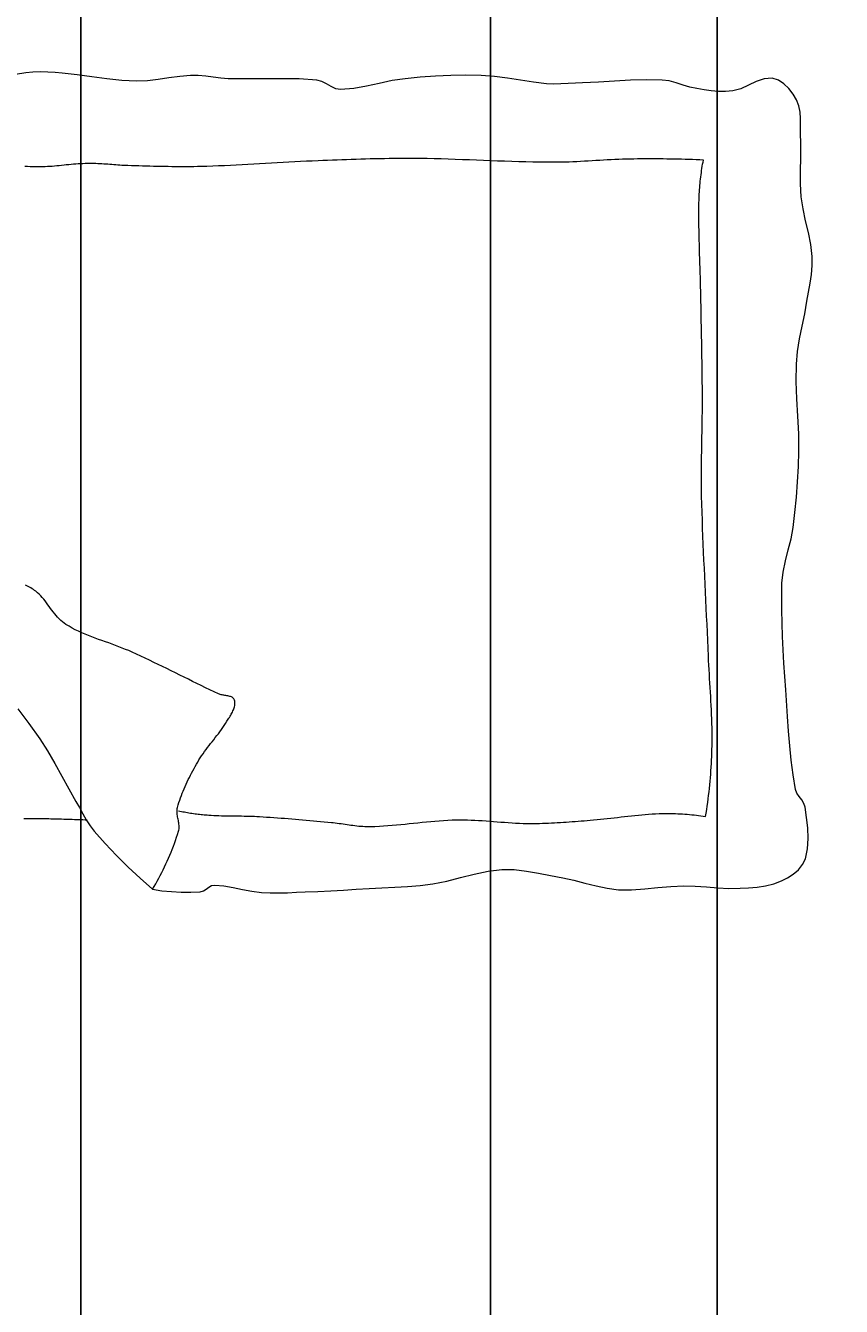
# Model space of a CAD drawing. Units: inches. Extents: x -15 to 423, y -713 to 71.
# Tile 8 of 24: x 70 to 144, y -234 to -117. Entities that reach past the tile are written whole.
import ezdxf

# ---------------------------------------------------------------- set-up
doc = ezdxf.new("R2010")
doc.units = ezdxf.units.IN
doc.header["$MEASUREMENT"] = 0
doc.layers.add('A-ANNO-DIMS', color=2, linetype='Continuous', lineweight=18)
doc.layers.add('A-FURN', color=9, linetype='Continuous', lineweight=13)
doc.styles.get("Standard").update_dxf_attribs({"font": 'arial.ttf'})
doc.dimstyles.get("Standard").update_dxf_attribs({"dimtxt": 0.18, "dimasz": 0.18, "dimexe": 0.18, "dimexo": 0.0625, "dimgap": 0.09, "dimtad": 0, "dimtih": 1, "dimtoh": 1, "dimdec": 0, "dimzin": 0, "dimdsep": 46, "dimlunit": 3, "dimtxsty": 'Standard', "dimcen": 0.09, "dimadec": 0, "dimazin": 0, "dimtfac": 1, "dimtdec": 0, "dimtofl": 0, "dimtmove": 0, "dimatfit": 3, "dimfxl": 1, "dimtolj": 1, "dimtzin": 0, "dimarcsym": 0})

# ---------------------------------------------------------------- blocks, each defined once
blk = doc.blocks.new('*D39')
at = {"layer": 'A-ANNO-DIMS', "color": 0, "lineweight": -2, "transparency": 16777216}
for p, q in [((75.05, -253.53), (75.05, 57.43)), ((75.23, 57.25), (93.19, 57.25)), ((112.22, 57.25), (94.26, 57.25)), ((112.4, -253.53), (112.4, 57.43))]:
    blk.add_line(p, q, dxfattribs=at)
at = {"layer": 'A-ANNO-DIMS', "color": 0, "transparency": 16777216}
for points in [[(75.23, 57.28), (75.23, 57.22), (75.05, 57.25)], [(112.22, 57.28), (112.22, 57.22), (112.4, 57.25)]]:
    blk.add_solid(points, dxfattribs=at)
at = {"layer": 'Defpoints', "color": 0, "transparency": 16777216}
for p in [(112.4, 57.25), (75.05, -253.59), (112.4, -253.59)]:
    blk.add_point(p, dxfattribs=at)
at = {"layer": 'A-ANNO-DIMS', "color": 0, "transparency": 16777216, "insert": (93.72, 57.25), "char_height": 0.18, "attachment_point": 5}
blk.add_mtext('\\A1;3\'-1 1/2"', dxfattribs=at)
blk = doc.blocks.new('*D42')
at = {"layer": 'A-ANNO-DIMS', "color": 0, "lineweight": -2, "transparency": 16777216}
for p, q in [((133.08, -409.94), (133.08, 57.43)), ((133.26, 57.25), (157.25, 57.25)), ((181.9, 57.25), (157.91, 57.25)), ((182.08, -409.94), (182.08, 57.43))]:
    blk.add_line(p, q, dxfattribs=at)
at = {"layer": 'A-ANNO-DIMS', "color": 0, "transparency": 16777216}
for points in [[(133.26, 57.28), (133.26, 57.22), (133.08, 57.25)], [(181.9, 57.28), (181.9, 57.22), (182.08, 57.25)]]:
    blk.add_solid(points, dxfattribs=at)
at = {"layer": 'Defpoints', "color": 0, "transparency": 16777216}
for p in [(182.08, 57.25), (133.08, -410), (182.08, -410)]:
    blk.add_point(p, dxfattribs=at)
at = {"layer": 'A-ANNO-DIMS', "color": 0, "transparency": 16777216, "insert": (157.58, 57.25), "char_height": 0.18, "attachment_point": 5}
blk.add_mtext('\\A1;4\'-1"', dxfattribs=at)

msp = doc.modelspace()

# ---------------------------------------------------------------- linework, layer by layer
at = {"layer": 'A-FURN'}
for p, q in [((70.02, -121.16), (69.09, -121.33)), ((70.68, -121.1), (70.02, -121.16)), ((71.35, -121.08), (70.68, -121.1)), ((72.02, -121.11), (71.35, -121.08)), ((72.69, -121.15), (72.02, -121.11)), ((73.35, -121.2), (72.69, -121.15)), ((74.71, -121.34), (73.35, -121.2)), ((76.06, -121.53), (74.71, -121.34)), ((85.06, -121.41), (84.07, -121.49)), ((85.74, -121.42), (85.06, -121.41)), ((86.43, -121.48), (85.74, -121.42)), ((107.39, -121.47), (106, -121.57)), ((108.78, -121.4), (107.39, -121.47)), ((110.17, -121.38), (108.78, -121.4)), ((111.57, -121.4), (110.17, -121.38)), ((112.76, -121.5), (111.57, -121.4)), ((77.41, -121.71), (76.06, -121.53)), ((78.77, -121.87), (77.41, -121.71)), ((80.13, -121.94), (78.77, -121.87)), ((81.12, -121.9), (80.13, -121.94)), ((82.1, -121.78), (81.12, -121.9)), ((83.08, -121.63), (82.1, -121.78)), ((84.07, -121.49), (83.08, -121.63)), ((87.11, -121.57), (86.43, -121.48)), ((87.8, -121.65), (87.11, -121.57)), ((88.48, -121.7), (87.8, -121.65)), ((90.1, -121.72), (88.48, -121.7)), ((91.72, -121.71), (90.1, -121.72)), ((93.34, -121.7), (91.72, -121.71)), ((94.95, -121.72), (93.34, -121.7)), ((96.56, -121.83), (94.95, -121.72)), ((97.01, -121.95), (96.56, -121.83)), ((97.44, -122.17), (97.01, -121.95)), ((97.86, -122.42), (97.44, -122.17)), ((98.29, -122.62), (97.86, -122.42)), ((98.74, -122.7), (98.29, -122.62)), ((99.93, -122.6), (98.74, -122.7)), ((101.1, -122.39), (99.93, -122.6)), ((102.26, -122.13), (101.1, -122.39)), ((103.43, -121.87), (102.26, -122.13)), ((104.61, -121.7), (103.43, -121.87)), ((106, -121.57), (104.61, -121.7)), ((113.95, -121.66), (112.76, -121.5)), ((115.13, -121.85), (113.95, -121.66)), ((116.32, -122.03), (115.13, -121.85)), ((117.52, -122.16), (116.32, -122.03)), ((118.17, -122.19), (117.52, -122.16)), ((118.83, -122.18), (118.17, -122.19)), ((119.49, -122.15), (118.83, -122.18)), ((120.15, -122.11), (119.49, -122.15)), ((120.81, -122.08), (120.15, -122.11)), ((122.26, -122.01), (120.81, -122.08)), ((123.71, -121.92), (122.26, -122.01)), ((125.16, -121.84), (123.71, -121.92)), ((126.6, -121.8), (125.16, -121.84)), ((128.05, -121.82), (126.6, -121.8)), ((128.7, -121.91), (128.05, -121.82)), ((129.34, -122.08), (128.7, -121.91)), ((129.97, -122.28), (129.34, -122.08)), ((130.6, -122.47), (129.97, -122.28)), ((131.24, -122.61), (130.6, -122.47)), ((131.89, -122.71), (131.24, -122.61)), ((135.24, -122.62), (134.5, -122.82)), ((135.95, -122.29), (135.24, -122.62)), ((136.65, -121.95), (135.95, -122.29)), ((137.37, -121.7), (136.65, -121.95)), ((138.1, -121.66), (137.37, -121.7)), ((138.66, -121.83), (138.1, -121.66)), ((139.17, -122.16), (138.66, -121.83)), ((139.63, -122.6), (139.17, -122.16)), ((140.01, -123.1), (139.63, -122.6)), ((132.54, -122.8), (131.89, -122.71)), ((133.2, -122.86), (132.54, -122.8)), ((133.85, -122.87), (133.2, -122.86)), ((134.5, -122.82), (133.85, -122.87)), ((140.33, -123.63), (140.01, -123.1)), ((140.54, -124.17), (140.33, -123.63)), ((140.64, -124.74), (140.54, -124.17)), ((140.68, -125.34), (140.64, -124.74)), ((140.68, -125.95), (140.68, -125.34)), ((140.69, -126.54), (140.68, -125.95)), ((140.71, -127.73), (140.69, -126.54)), ((140.7, -128.92), (140.71, -127.73)), ((73.08, -129.64), (72.86, -129.66)), ((73.29, -129.62), (73.08, -129.64)), ((73.51, -129.59), (73.29, -129.62)), ((73.72, -129.57), (73.51, -129.59)), ((73.94, -129.55), (73.72, -129.57)), ((74.15, -129.53), (73.94, -129.55)), ((74.37, -129.51), (74.15, -129.53)), ((74.59, -129.49), (74.37, -129.51)), ((74.8, -129.47), (74.59, -129.49)), ((75.02, -129.46), (74.8, -129.47)), ((75.23, -129.45), (75.02, -129.46)), ((75.45, -129.44), (75.23, -129.45)), ((75.67, -129.43), (75.45, -129.44)), ((75.85, -129.43), (75.67, -129.43)), ((76.03, -129.43), (75.85, -129.43)), ((76.22, -129.44), (76.03, -129.43)), ((76.4, -129.44), (76.22, -129.44)), ((76.58, -129.45), (76.4, -129.44)), ((76.77, -129.46), (76.58, -129.45)), ((76.95, -129.47), (76.77, -129.46)), ((77.13, -129.49), (76.95, -129.47)), ((77.32, -129.5), (77.13, -129.49)), ((77.5, -129.51), (77.32, -129.5)), ((77.69, -129.53), (77.5, -129.51)), ((77.87, -129.54), (77.69, -129.53)), ((78.05, -129.56), (77.87, -129.54)), ((78.24, -129.57), (78.05, -129.56)), ((78.42, -129.58), (78.24, -129.57)), ((78.6, -129.6), (78.42, -129.58)), ((78.79, -129.61), (78.6, -129.6)), ((78.97, -129.62), (78.79, -129.61)), ((79.15, -129.63), (78.97, -129.62)), ((79.34, -129.63), (79.15, -129.63)), ((79.67, -129.64), (79.34, -129.63)), ((80, -129.65), (79.67, -129.64)), ((88.15, -129.64), (87.61, -129.66)), ((88.68, -129.62), (88.15, -129.64)), ((89.22, -129.59), (88.68, -129.62)), ((89.75, -129.56), (89.22, -129.59)), ((90.28, -129.53), (89.75, -129.56)), ((90.82, -129.5), (90.28, -129.53)), ((91.35, -129.47), (90.82, -129.5)), ((91.88, -129.44), (91.35, -129.47)), ((92.42, -129.41), (91.88, -129.44)), ((92.95, -129.38), (92.42, -129.41)), ((93.49, -129.35), (92.95, -129.38)), ((94.02, -129.32), (93.49, -129.35)), ((94.55, -129.29), (94.02, -129.32)), ((95.09, -129.26), (94.55, -129.29)), ((95.62, -129.23), (95.09, -129.26)), ((96.15, -129.21), (95.62, -129.23)), ((96.69, -129.19), (96.15, -129.21)), ((97.12, -129.17), (96.69, -129.19)), ((97.55, -129.16), (97.12, -129.17)), ((97.99, -129.14), (97.55, -129.16)), ((98.42, -129.12), (97.99, -129.14)), ((98.85, -129.11), (98.42, -129.12)), ((99.28, -129.09), (98.85, -129.11)), ((99.71, -129.08), (99.28, -129.09)), ((100.15, -129.06), (99.71, -129.08)), ((100.58, -129.05), (100.15, -129.06)), ((101.01, -129.04), (100.58, -129.05)), ((101.44, -129.02), (101.01, -129.04)), ((101.88, -129.01), (101.44, -129.02)), ((102.31, -129), (101.88, -129.01)), ((102.74, -129), (102.31, -129)), ((103.17, -128.99), (102.74, -129)), ((103.6, -128.98), (103.17, -128.99)), ((104.04, -128.98), (103.6, -128.98)), ((104.47, -128.98), (104.04, -128.98)), ((104.9, -128.98), (104.47, -128.98)), ((105.33, -128.98), (104.9, -128.98)), ((105.98, -128.98), (105.33, -128.98)), ((106.62, -128.99), (105.98, -128.98)), ((107.26, -129.01), (106.62, -128.99)), ((107.91, -129.02), (107.26, -129.01)), ((108.55, -129.04), (107.91, -129.02)), ((109.19, -129.06), (108.55, -129.04)), ((109.84, -129.09), (109.19, -129.06)), ((110.48, -129.11), (109.84, -129.09)), ((111.12, -129.13), (110.48, -129.11)), ((111.76, -129.16), (111.12, -129.13)), ((112.41, -129.18), (111.76, -129.16)), ((113.05, -129.21), (112.41, -129.18)), ((113.69, -129.23), (113.05, -129.21)), ((114.34, -129.25), (113.69, -129.23)), ((114.98, -129.27), (114.34, -129.25)), ((115.62, -129.29), (114.98, -129.27)), ((116.26, -129.3), (115.62, -129.29)), ((116.91, -129.31), (116.26, -129.3)), ((117.55, -129.32), (116.91, -129.31)), ((118.19, -129.32), (117.55, -129.32)), ((118.54, -129.32), (118.19, -129.32)), ((118.89, -129.32), (118.54, -129.32)), ((119.24, -129.31), (118.89, -129.32)), ((119.59, -129.3), (119.24, -129.31)), ((119.93, -129.29), (119.59, -129.3)), ((120.28, -129.27), (119.93, -129.29)), ((120.63, -129.25), (120.28, -129.27)), ((120.98, -129.23), (120.63, -129.25)), ((121.32, -129.21), (120.98, -129.23)), ((121.67, -129.19), (121.32, -129.21)), ((122.02, -129.17), (121.67, -129.19)), ((122.37, -129.15), (122.02, -129.17)), ((122.71, -129.13), (122.37, -129.15)), ((123.06, -129.11), (122.71, -129.13)), ((123.41, -129.09), (123.06, -129.11)), ((123.76, -129.08), (123.41, -129.09)), ((124.11, -129.06), (123.76, -129.08)), ((124.45, -129.05), (124.11, -129.06)), ((124.8, -129.04), (124.45, -129.05)), ((125.15, -129.03), (124.8, -129.04)), ((125.48, -129.03), (125.15, -129.03)), ((125.82, -129.02), (125.48, -129.03)), ((126.15, -129.02), (125.82, -129.02)), ((126.48, -129.02), (126.15, -129.02)), ((126.82, -129.02), (126.48, -129.02)), ((127.15, -129.02), (126.82, -129.02)), ((127.49, -129.02), (127.15, -129.02)), ((127.82, -129.02), (127.49, -129.02)), ((128.15, -129.02), (127.82, -129.02)), ((128.49, -129.03), (128.15, -129.02)), ((128.82, -129.03), (128.49, -129.03)), ((129.15, -129.04), (128.82, -129.03)), ((129.49, -129.04), (129.15, -129.04)), ((129.82, -129.05), (129.49, -129.04)), ((130.16, -129.06), (129.82, -129.05)), ((130.49, -129.07), (130.16, -129.06)), ((130.82, -129.08), (130.49, -129.07)), ((131.16, -129.09), (130.82, -129.08)), ((131.49, -129.1), (131.16, -129.09)), ((131.82, -129.12), (131.49, -129.1)), ((131.72, -129.69), (131.75, -129.5)), ((131.75, -129.5), (131.79, -129.31)), ((131.79, -129.31), (131.82, -129.12)), ((140.68, -130.1), (140.7, -128.92)), ((70.18, -129.72), (69.95, -129.71)), ((70.42, -129.73), (70.18, -129.72)), ((70.65, -129.74), (70.42, -129.73)), ((70.88, -129.74), (70.65, -129.74)), ((71.12, -129.74), (70.88, -129.74)), ((71.35, -129.74), (71.12, -129.74)), ((71.56, -129.74), (71.35, -129.74)), ((71.78, -129.73), (71.56, -129.74)), ((72, -129.72), (71.78, -129.73)), ((72.21, -129.71), (72, -129.72)), ((72.43, -129.7), (72.21, -129.71)), ((72.64, -129.68), (72.43, -129.7)), ((72.86, -129.66), (72.64, -129.68)), ((80.34, -129.66), (80, -129.65)), ((80.67, -129.67), (80.34, -129.66)), ((81.01, -129.68), (80.67, -129.67)), ((81.34, -129.69), (81.01, -129.68)), ((81.67, -129.7), (81.34, -129.69)), ((82.01, -129.71), (81.67, -129.7)), ((82.34, -129.71), (82.01, -129.71)), ((82.67, -129.72), (82.34, -129.71)), ((83.01, -129.72), (82.67, -129.72)), ((83.34, -129.73), (83.01, -129.72)), ((83.68, -129.73), (83.34, -129.73)), ((84.01, -129.74), (83.68, -129.73)), ((84.34, -129.74), (84.01, -129.74)), ((84.68, -129.74), (84.34, -129.74)), ((85.01, -129.73), (84.68, -129.74)), ((85.34, -129.73), (85.01, -129.73)), ((85.68, -129.72), (85.34, -129.73)), ((86.01, -129.72), (85.68, -129.72)), ((86.55, -129.7), (86.01, -129.72)), ((87.08, -129.68), (86.55, -129.7)), ((87.61, -129.66), (87.08, -129.68)), ((131.56, -130.85), (131.59, -130.66)), ((131.59, -130.66), (131.61, -130.47)), ((131.61, -130.47), (131.64, -130.27)), ((131.64, -130.27), (131.66, -130.08)), ((131.66, -130.08), (131.69, -129.89)), ((131.69, -129.89), (131.72, -129.69)), ((140.68, -131.29), (140.68, -130.1)), ((131.46, -132.02), (131.48, -131.83)), ((131.48, -131.83), (131.49, -131.63)), ((131.49, -131.63), (131.51, -131.44)), ((131.51, -131.44), (131.52, -131.24)), ((131.52, -131.24), (131.54, -131.05)), ((131.54, -131.05), (131.56, -130.85)), ((140.75, -132.47), (140.68, -131.29)), ((131.42, -133), (131.43, -132.8)), ((131.42, -133.42), (131.42, -133)), ((131.43, -132.61), (131.44, -132.41)), ((131.43, -132.8), (131.43, -132.61)), ((131.44, -132.41), (131.45, -132.22)), ((131.45, -132.22), (131.46, -132.02)), ((140.91, -133.57), (140.75, -132.47)), ((131.41, -133.85), (131.42, -133.42)), ((131.41, -134.28), (131.41, -133.85)), ((131.42, -134.7), (131.41, -134.28)), ((141.15, -134.66), (140.91, -133.57)), ((131.42, -135.13), (131.42, -134.7)), ((131.43, -135.56), (131.42, -135.13)), ((141.4, -135.74), (141.15, -134.66)), ((131.44, -135.98), (131.43, -135.56)), ((131.45, -136.41), (131.44, -135.98)), ((131.46, -136.83), (131.45, -136.41)), ((141.62, -136.83), (141.4, -135.74)), ((131.47, -137.26), (131.46, -136.83)), ((131.48, -137.69), (131.47, -137.26)), ((131.5, -138.11), (131.48, -137.69)), ((141.75, -137.93), (141.62, -136.83)), ((131.51, -138.54), (131.5, -138.11)), ((131.52, -138.96), (131.51, -138.54)), ((131.54, -139.39), (131.52, -138.96)), ((141.67, -139.55), (141.75, -138.74)), ((141.75, -138.74), (141.75, -137.93)), ((131.55, -139.82), (131.54, -139.39)), ((131.56, -140.24), (131.55, -139.82)), ((141.55, -140.36), (141.67, -139.55)), ((131.57, -140.67), (131.56, -140.24)), ((131.58, -141.09), (131.57, -140.67)), ((131.59, -141.52), (131.58, -141.09)), ((141.27, -141.98), (141.4, -141.17)), ((141.4, -141.17), (141.55, -140.36)), ((131.6, -141.98), (131.59, -141.52)), ((131.61, -142.44), (131.6, -141.98)), ((131.62, -142.9), (131.61, -142.44)), ((141.07, -143.13), (141.27, -141.98)), ((131.62, -143.37), (131.62, -142.9)), ((131.63, -143.83), (131.62, -143.37)), ((140.84, -144.27), (141.07, -143.13)), ((131.64, -144.29), (131.63, -143.83)), ((131.65, -144.75), (131.64, -144.29)), ((131.66, -145.21), (131.65, -144.75)), ((140.6, -145.42), (140.84, -144.27)), ((131.67, -145.67), (131.66, -145.21)), ((131.68, -146.13), (131.67, -145.67)), ((140.41, -146.57), (140.6, -145.42)), ((131.68, -146.59), (131.68, -146.13)), ((131.69, -147.06), (131.68, -146.59)), ((131.7, -147.52), (131.69, -147.06)), ((140.3, -147.72), (140.41, -146.57)), ((131.71, -147.98), (131.7, -147.52)), ((131.71, -148.44), (131.71, -147.98)), ((140.27, -149.31), (140.3, -147.72)), ((131.72, -148.9), (131.71, -148.44)), ((131.72, -149.36), (131.72, -148.9)), ((131.73, -149.82), (131.72, -149.36)), ((140.34, -150.9), (140.27, -149.31)), ((131.73, -150.28), (131.73, -149.82)), ((131.73, -150.74), (131.73, -150.28)), ((131.73, -151.2), (131.73, -150.74)), ((131.73, -151.65), (131.73, -151.2)), ((131.73, -152.1), (131.73, -151.65)), ((140.43, -152.49), (140.34, -150.9)), ((131.71, -153.45), (131.72, -153)), ((131.72, -152.55), (131.73, -152.1)), ((131.72, -153), (131.72, -152.55)), ((140.52, -154.08), (140.43, -152.49)), ((131.69, -154.35), (131.7, -153.9)), ((131.7, -153.9), (131.71, -153.45)), ((140.53, -155.67), (140.52, -154.08)), ((131.67, -155.71), (131.68, -155.26)), ((131.68, -154.81), (131.69, -154.35)), ((131.68, -155.26), (131.68, -154.81)), ((131.65, -156.61), (131.66, -156.16)), ((131.66, -156.16), (131.67, -155.71)), ((140.49, -157.07), (140.53, -155.67)), ((131.65, -157.06), (131.65, -156.61)), ((131.65, -157.51), (131.65, -157.06)), ((131.65, -157.96), (131.65, -157.51)), ((140.41, -158.47), (140.49, -157.07)), ((131.65, -158.41), (131.65, -157.96)), ((131.65, -158.87), (131.65, -158.41)), ((140.3, -159.86), (140.41, -158.47)), ((131.65, -159.32), (131.65, -158.87)), ((131.66, -159.77), (131.65, -159.32)), ((131.68, -160.5), (131.66, -159.77)), ((140.17, -161.25), (140.3, -159.86)), ((131.7, -161.23), (131.68, -160.5)), ((131.73, -161.96), (131.7, -161.23)), ((131.75, -162.69), (131.73, -161.96)), ((140, -162.64), (140.17, -161.25)), ((131.78, -163.42), (131.75, -162.69)), ((131.81, -164.14), (131.78, -163.42)), ((139.82, -163.66), (140, -162.64)), ((131.84, -164.87), (131.81, -164.14)), ((139.31, -165.68), (139.57, -164.67)), ((139.57, -164.67), (139.82, -163.66)), ((131.87, -165.6), (131.84, -164.87)), ((131.91, -166.33), (131.87, -165.6)), ((139.1, -166.69), (139.31, -165.68)), ((131.94, -167.06), (131.91, -166.33)), ((138.99, -167.71), (139.1, -166.69)), ((70.12, -167.94), (70, -167.88)), ((70.25, -168), (70.12, -167.94)), ((70.37, -168.07), (70.25, -168)), ((70.49, -168.13), (70.37, -168.07)), ((70.6, -168.21), (70.49, -168.13)), ((131.98, -167.79), (131.94, -167.06)), ((132.01, -168.52), (131.98, -167.79)), ((138.97, -170.14), (138.99, -167.71)), ((70.72, -168.28), (70.6, -168.21)), ((70.83, -168.36), (70.72, -168.28)), ((70.94, -168.44), (70.83, -168.36)), ((71.1, -168.58), (70.94, -168.44)), ((71.25, -168.72), (71.1, -168.58)), ((71.39, -168.86), (71.25, -168.72)), ((71.53, -169.02), (71.39, -168.86)), ((71.66, -169.17), (71.53, -169.02)), ((71.79, -169.33), (71.66, -169.17)), ((71.91, -169.5), (71.79, -169.33)), ((132.05, -169.25), (132.01, -168.52)), ((132.08, -169.98), (132.05, -169.25)), ((72.04, -169.67), (71.91, -169.5)), ((72.16, -169.83), (72.04, -169.67)), ((72.28, -170), (72.16, -169.83)), ((72.41, -170.17), (72.28, -170)), ((72.53, -170.33), (72.41, -170.17)), ((72.66, -170.5), (72.53, -170.33)), ((72.79, -170.65), (72.66, -170.5)), ((132.12, -170.71), (132.08, -169.98)), ((139.04, -172.57), (138.97, -170.14)), ((72.93, -170.81), (72.79, -170.65)), ((73.07, -170.95), (72.93, -170.81)), ((73.21, -171.1), (73.07, -170.95)), ((73.36, -171.23), (73.21, -171.1)), ((73.52, -171.35), (73.36, -171.23)), ((73.69, -171.47), (73.52, -171.35)), ((73.97, -171.64), (73.69, -171.47)), ((74.26, -171.8), (73.97, -171.64)), ((132.16, -171.44), (132.12, -170.71)), ((132.19, -172.17), (132.16, -171.44)), ((74.54, -171.95), (74.26, -171.8)), ((74.84, -172.09), (74.54, -171.95)), ((75.13, -172.23), (74.84, -172.09)), ((75.43, -172.36), (75.13, -172.23)), ((75.74, -172.48), (75.43, -172.36)), ((76.04, -172.6), (75.74, -172.48)), ((76.35, -172.72), (76.04, -172.6)), ((76.66, -172.83), (76.35, -172.72)), ((76.97, -172.94), (76.66, -172.83)), ((132.22, -172.9), (132.19, -172.17)), ((139.17, -175), (139.04, -172.57)), ((77.28, -173.05), (76.97, -172.94)), ((77.59, -173.16), (77.28, -173.05)), ((77.9, -173.27), (77.59, -173.16)), ((78.21, -173.38), (77.9, -173.27)), ((78.51, -173.5), (78.21, -173.38)), ((78.82, -173.62), (78.51, -173.5)), ((79.13, -173.74), (78.82, -173.62)), ((79.43, -173.86), (79.13, -173.74)), ((79.73, -174), (79.43, -173.86)), ((80.12, -174.18), (79.73, -174)), ((132.26, -173.63), (132.22, -172.9)), ((132.29, -174.35), (132.26, -173.63)), ((80.52, -174.36), (80.12, -174.18)), ((80.92, -174.55), (80.52, -174.36)), ((81.31, -174.74), (80.92, -174.55)), ((81.71, -174.93), (81.31, -174.74)), ((82.1, -175.12), (81.71, -174.93)), ((82.49, -175.31), (82.1, -175.12)), ((132.3, -174.76), (132.29, -174.35)), ((132.32, -175.17), (132.3, -174.76)), ((132.35, -175.58), (132.32, -175.17)), ((139.33, -177.43), (139.17, -175)), ((82.89, -175.5), (82.49, -175.31)), ((83.28, -175.69), (82.89, -175.5)), ((83.67, -175.89), (83.28, -175.69)), ((84.06, -176.08), (83.67, -175.89)), ((84.46, -176.27), (84.06, -176.08)), ((84.85, -176.47), (84.46, -176.27)), ((132.37, -175.99), (132.35, -175.58)), ((132.39, -176.4), (132.37, -175.99)), ((85.24, -176.66), (84.85, -176.47)), ((85.63, -176.85), (85.24, -176.66)), ((86.03, -177.05), (85.63, -176.85)), ((86.42, -177.24), (86.03, -177.05)), ((86.81, -177.43), (86.42, -177.24)), ((87.21, -177.61), (86.81, -177.43)), ((132.42, -176.81), (132.39, -176.4)), ((132.44, -177.22), (132.42, -176.81)), ((132.46, -177.63), (132.44, -177.22)), ((139.5, -179.85), (139.33, -177.43)), ((87.61, -177.8), (87.21, -177.61)), ((87.68, -177.83), (87.61, -177.8)), ((87.76, -177.86), (87.68, -177.83)), ((87.84, -177.88), (87.76, -177.86)), ((87.92, -177.9), (87.84, -177.88)), ((88.01, -177.92), (87.92, -177.9)), ((88.1, -177.93), (88.01, -177.92)), ((88.19, -177.94), (88.1, -177.93)), ((88.28, -177.96), (88.19, -177.94)), ((88.37, -177.97), (88.28, -177.96)), ((88.45, -177.99), (88.37, -177.97)), ((88.54, -178.01), (88.45, -177.99)), ((88.62, -178.03), (88.54, -178.01)), ((88.7, -178.05), (88.62, -178.03)), ((88.77, -178.08), (88.7, -178.05)), ((88.84, -178.11), (88.77, -178.08)), ((88.9, -178.15), (88.84, -178.11)), ((88.95, -178.2), (88.9, -178.15)), ((89, -178.25), (88.95, -178.2)), ((89.03, -178.31), (89, -178.25)), ((89.06, -178.38), (89.03, -178.31)), ((89.09, -178.48), (89.06, -178.38)), ((89.1, -178.58), (89.09, -178.48)), ((89.1, -178.68), (89.1, -178.58)), ((89.1, -178.78), (89.1, -178.68)), ((132.49, -178.04), (132.46, -177.63)), ((132.51, -178.45), (132.49, -178.04)), ((132.53, -178.86), (132.51, -178.45)), ((69.29, -179.17), (70.31, -180.51)), ((88.59, -179.94), (88.65, -179.84)), ((88.65, -179.84), (88.71, -179.75)), ((88.71, -179.75), (88.76, -179.65)), ((88.76, -179.65), (88.82, -179.56)), ((88.82, -179.56), (88.87, -179.46)), ((88.87, -179.46), (88.92, -179.36)), ((88.92, -179.36), (88.96, -179.27)), ((88.96, -179.27), (89, -179.17)), ((89, -179.17), (89.04, -179.07)), ((89.04, -179.07), (89.06, -178.97)), ((89.06, -178.97), (89.08, -178.87)), ((89.08, -178.87), (89.1, -178.78)), ((132.55, -179.27), (132.53, -178.86)), ((132.57, -179.68), (132.55, -179.27)), ((132.58, -180.09), (132.57, -179.68)), ((139.59, -181.19), (139.5, -179.85)), ((70.31, -180.51), (71.29, -181.89)), ((87.86, -181.06), (87.99, -180.87)), ((87.99, -180.87), (88.12, -180.68)), ((88.12, -180.68), (88.25, -180.49)), ((88.25, -180.49), (88.37, -180.3)), ((88.37, -180.3), (88.42, -180.21)), ((88.42, -180.21), (88.48, -180.12)), ((88.48, -180.12), (88.53, -180.03)), ((88.53, -180.03), (88.59, -179.94)), ((132.6, -180.5), (132.58, -180.09)), ((132.61, -180.91), (132.6, -180.5)), ((132.61, -181.32), (132.61, -180.91)), ((71.29, -181.89), (72, -183)), ((86.88, -182.34), (87.02, -182.16)), ((87.02, -182.16), (87.17, -181.98)), ((87.17, -181.98), (87.31, -181.79)), ((87.31, -181.79), (87.45, -181.61)), ((87.45, -181.61), (87.59, -181.43)), ((87.59, -181.43), (87.73, -181.25)), ((87.73, -181.25), (87.86, -181.06)), ((132.62, -181.72), (132.61, -181.32)), ((132.61, -182.13), (132.62, -181.72)), ((132.61, -182.54), (132.61, -182.13)), ((139.7, -182.53), (139.59, -181.19)), ((72, -183), (72.66, -184.15)), ((86.06, -183.44), (86.19, -183.26)), ((86.19, -183.26), (86.33, -183.07)), ((86.33, -183.07), (86.46, -182.88)), ((86.46, -182.88), (86.6, -182.7)), ((86.6, -182.7), (86.74, -182.52)), ((86.74, -182.52), (86.88, -182.34)), ((132.58, -183.51), (132.59, -183.19)), ((132.59, -183.19), (132.6, -182.87)), ((132.6, -182.87), (132.61, -182.54)), ((139.83, -183.86), (139.7, -182.53)), ((72.66, -184.15), (73.31, -185.3)), ((85.37, -184.62), (85.47, -184.42)), ((85.47, -184.42), (85.59, -184.22)), ((85.59, -184.22), (85.7, -184.03)), ((85.7, -184.03), (85.81, -183.83)), ((85.81, -183.83), (85.94, -183.64)), ((85.94, -183.64), (86.06, -183.44)), ((132.51, -184.81), (132.53, -184.48)), ((132.53, -184.48), (132.55, -184.16)), ((132.55, -184.16), (132.57, -183.84)), ((132.57, -183.84), (132.58, -183.51)), ((140.01, -185.19), (139.83, -183.86)), ((73.31, -185.3), (73.94, -186.46)), ((84.74, -185.83), (84.84, -185.62)), ((84.84, -185.62), (84.94, -185.42)), ((84.94, -185.42), (85.05, -185.22)), ((85.05, -185.22), (85.15, -185.02)), ((85.15, -185.02), (85.26, -184.82)), ((85.26, -184.82), (85.37, -184.62)), ((132.43, -185.77), (132.46, -185.45)), ((132.46, -185.45), (132.49, -185.13)), ((132.49, -185.13), (132.51, -184.81)), ((140.23, -186.51), (140.01, -185.19)), ((73.94, -186.46), (74.6, -187.61)), ((84.21, -187.08), (84.29, -186.87)), ((84.29, -186.87), (84.38, -186.66)), ((84.38, -186.66), (84.47, -186.45)), ((84.47, -186.45), (84.56, -186.24)), ((84.56, -186.24), (84.65, -186.03)), ((84.65, -186.03), (84.74, -185.83)), ((132.3, -187.06), (132.34, -186.74)), ((132.34, -186.74), (132.37, -186.42)), ((132.37, -186.42), (132.4, -186.1)), ((132.4, -186.1), (132.43, -185.77)), ((140.36, -186.85), (140.23, -186.51)), ((140.56, -187.17), (140.36, -186.85)), ((74.6, -187.61), (74.92, -188.17)), ((83.86, -188.15), (83.92, -187.93)), ((83.92, -187.93), (83.99, -187.72)), ((83.99, -187.72), (84.06, -187.5)), ((84.06, -187.5), (84.13, -187.29)), ((84.13, -187.29), (84.21, -187.08)), ((132.13, -188.35), (132.17, -188.03)), ((132.17, -188.03), (132.22, -187.7)), ((132.22, -187.7), (132.26, -187.38)), ((132.26, -187.38), (132.3, -187.06)), ((140.79, -187.47), (140.56, -187.17)), ((140.99, -187.79), (140.79, -187.47)), ((141.1, -188.14), (140.99, -187.79)), ((70.03, -189.19), (69.84, -189.19)), ((70.22, -189.19), (70.03, -189.19)), ((70.4, -189.19), (70.22, -189.19)), ((70.59, -189.19), (70.4, -189.19)), ((70.78, -189.2), (70.59, -189.19)), ((70.97, -189.2), (70.78, -189.2)), ((71.15, -189.2), (70.97, -189.2)), ((71.34, -189.2), (71.15, -189.2)), ((71.53, -189.2), (71.34, -189.2)), ((71.72, -189.21), (71.53, -189.2)), ((71.91, -189.21), (71.72, -189.21)), ((74.92, -188.17), (75.22, -188.73)), ((75.22, -188.73), (75.54, -189.29)), ((83.82, -188.36), (83.84, -188.25)), ((83.82, -188.47), (83.82, -188.36)), ((83.82, -188.58), (83.82, -188.47)), ((83.82, -188.69), (83.82, -188.58)), ((83.84, -188.8), (83.82, -188.69)), ((83.84, -188.25), (83.86, -188.15)), ((83.85, -188.91), (83.84, -188.8)), ((83.87, -189.02), (83.85, -188.91)), ((83.89, -189.13), (83.87, -189.02)), ((83.92, -189.24), (83.89, -189.13)), ((83.94, -188.47), (84.08, -188.49)), ((84.08, -188.49), (84.22, -188.52)), ((84.22, -188.52), (84.35, -188.55)), ((84.35, -188.55), (84.49, -188.57)), ((84.49, -188.57), (84.63, -188.6)), ((84.63, -188.6), (84.77, -188.62)), ((84.77, -188.62), (84.9, -188.64)), ((84.9, -188.64), (85.04, -188.67)), ((85.04, -188.67), (85.18, -188.69)), ((85.18, -188.69), (85.32, -188.71)), ((85.32, -188.71), (85.46, -188.73)), ((85.46, -188.73), (85.6, -188.74)), ((85.6, -188.74), (85.74, -188.76)), ((85.74, -188.76), (85.87, -188.78)), ((85.87, -188.78), (86.01, -188.79)), ((86.01, -188.79), (86.15, -188.81)), ((86.15, -188.81), (86.29, -188.82)), ((86.29, -188.82), (86.43, -188.83)), ((86.43, -188.83), (86.57, -188.84)), ((86.57, -188.84), (86.71, -188.85)), ((86.71, -188.85), (86.94, -188.87)), ((86.94, -188.87), (87.17, -188.88)), ((87.17, -188.88), (87.4, -188.89)), ((87.4, -188.89), (87.63, -188.9)), ((87.63, -188.9), (87.86, -188.91)), ((87.86, -188.91), (88.09, -188.91)), ((88.09, -188.91), (88.33, -188.92)), ((88.33, -188.92), (88.56, -188.92)), ((88.56, -188.92), (88.79, -188.92)), ((88.79, -188.92), (89.02, -188.93)), ((89.02, -188.93), (89.25, -188.93)), ((89.25, -188.93), (89.48, -188.93)), ((89.48, -188.93), (89.71, -188.93)), ((89.71, -188.93), (89.94, -188.94)), ((89.94, -188.94), (90.17, -188.94)), ((90.17, -188.94), (90.4, -188.95)), ((90.4, -188.95), (90.64, -188.95)), ((90.64, -188.95), (90.87, -188.96)), ((90.87, -188.96), (91.1, -188.97)), ((91.1, -188.97), (91.33, -188.99)), ((91.33, -188.99), (91.66, -189.01)), ((91.66, -189.01), (91.98, -189.03)), ((91.98, -189.03), (92.31, -189.05)), ((92.31, -189.05), (92.64, -189.08)), ((92.64, -189.08), (92.97, -189.1)), ((92.97, -189.1), (93.3, -189.13)), ((93.3, -189.13), (93.63, -189.15)), ((93.63, -189.15), (93.95, -189.18)), ((93.95, -189.18), (94.28, -189.21)), ((94.28, -189.21), (94.61, -189.23)), ((122.43, -189.24), (122.75, -189.2)), ((122.75, -189.2), (123.06, -189.17)), ((123.06, -189.17), (123.37, -189.13)), ((123.37, -189.13), (123.69, -189.1)), ((123.69, -189.1), (124, -189.06)), ((124, -189.06), (124.32, -189.02)), ((124.32, -189.02), (124.63, -188.99)), ((124.63, -188.99), (124.94, -188.95)), ((124.94, -188.95), (125.26, -188.91)), ((125.26, -188.91), (125.57, -188.88)), ((125.57, -188.88), (125.89, -188.85)), ((125.89, -188.85), (126.2, -188.82)), ((126.2, -188.82), (126.52, -188.79)), ((126.52, -188.79), (126.83, -188.77)), ((126.83, -188.77), (127.15, -188.75)), ((127.15, -188.75), (127.46, -188.73)), ((127.46, -188.73), (127.78, -188.72)), ((127.78, -188.72), (127.99, -188.71)), ((127.99, -188.71), (128.2, -188.71)), ((128.2, -188.71), (128.41, -188.71)), ((128.41, -188.71), (128.63, -188.71)), ((128.63, -188.71), (128.84, -188.71)), ((128.84, -188.71), (129.05, -188.71)), ((129.05, -188.71), (129.27, -188.72)), ((129.27, -188.72), (129.48, -188.73)), ((129.48, -188.73), (129.69, -188.74)), ((129.69, -188.74), (129.91, -188.75)), ((129.91, -188.75), (130.12, -188.76)), ((130.12, -188.76), (130.33, -188.78)), ((130.33, -188.78), (130.55, -188.8)), ((130.55, -188.8), (130.76, -188.82)), ((130.76, -188.82), (130.97, -188.84)), ((130.97, -188.84), (131.18, -188.87)), ((131.18, -188.87), (131.39, -188.89)), ((131.39, -188.89), (131.6, -188.92)), ((131.6, -188.92), (131.81, -188.95)), ((131.81, -188.95), (132.03, -188.98)), ((132.03, -188.98), (132.08, -188.67)), ((132.08, -188.67), (132.13, -188.35)), ((141.23, -189.08), (141.1, -188.14)), ((141.34, -190.03), (141.23, -189.08)), ((72.11, -189.21), (71.91, -189.21)), ((72.3, -189.22), (72.11, -189.21)), ((72.5, -189.22), (72.3, -189.22)), ((72.69, -189.23), (72.5, -189.22)), ((72.89, -189.23), (72.69, -189.23)), ((73.09, -189.24), (72.89, -189.23)), ((73.28, -189.24), (73.09, -189.24)), ((73.48, -189.25), (73.28, -189.24)), ((73.67, -189.25), (73.48, -189.25)), ((73.87, -189.26), (73.67, -189.25)), ((74.06, -189.26), (73.87, -189.26)), ((74.26, -189.27), (74.06, -189.26)), ((74.46, -189.28), (74.26, -189.27)), ((74.65, -189.28), (74.46, -189.28)), ((74.85, -189.29), (74.65, -189.28)), ((75.04, -189.3), (74.85, -189.29)), ((75.24, -189.3), (75.04, -189.3)), ((75.44, -189.31), (75.24, -189.3)), ((75.63, -189.32), (75.44, -189.31)), ((75.54, -189.29), (75.88, -189.83)), ((75.88, -189.83), (76.27, -190.33)), ((76.27, -190.33), (77.27, -191.45)), ((83.87, -190.61), (83.96, -190.33)), ((83.94, -189.35), (83.92, -189.24)), ((83.96, -189.46), (83.94, -189.35)), ((83.98, -189.57), (83.96, -189.46)), ((83.96, -190.33), (83.98, -190.23)), ((83.99, -189.68), (83.98, -189.57)), ((83.98, -190.23), (84, -190.12)), ((84, -189.79), (83.99, -189.68)), ((84.01, -189.9), (84, -189.79)), ((84, -190.12), (84.01, -190.01)), ((84.01, -190.01), (84.01, -189.9)), ((94.61, -189.23), (94.94, -189.26)), ((94.94, -189.26), (95.27, -189.29)), ((95.27, -189.29), (95.59, -189.32)), ((95.59, -189.32), (95.92, -189.35)), ((95.92, -189.35), (96.25, -189.38)), ((96.25, -189.38), (96.58, -189.41)), ((96.58, -189.41), (96.91, -189.44)), ((96.91, -189.44), (97.23, -189.47)), ((97.23, -189.47), (97.56, -189.5)), ((97.56, -189.5), (97.89, -189.53)), ((97.89, -189.53), (98.07, -189.54)), ((98.07, -189.54), (98.25, -189.56)), ((98.25, -189.56), (98.43, -189.59)), ((98.43, -189.59), (98.61, -189.61)), ((98.61, -189.61), (98.79, -189.63)), ((98.79, -189.63), (98.97, -189.66)), ((98.97, -189.66), (99.15, -189.68)), ((99.15, -189.68), (99.33, -189.71)), ((99.33, -189.71), (99.51, -189.73)), ((99.51, -189.73), (99.68, -189.76)), ((99.68, -189.76), (99.86, -189.78)), ((99.86, -189.78), (100.04, -189.81)), ((100.04, -189.81), (100.22, -189.83)), ((100.22, -189.83), (100.4, -189.85)), ((100.4, -189.85), (100.58, -189.86)), ((100.58, -189.86), (100.76, -189.87)), ((100.76, -189.87), (100.94, -189.88)), ((100.94, -189.88), (101.12, -189.89)), ((101.12, -189.89), (101.3, -189.89)), ((101.3, -189.89), (101.48, -189.89)), ((101.48, -189.89), (101.87, -189.88)), ((101.87, -189.88), (102.27, -189.86)), ((102.27, -189.86), (102.66, -189.84)), ((102.66, -189.84), (103.05, -189.81)), ((103.05, -189.81), (103.44, -189.78)), ((103.44, -189.78), (103.83, -189.75)), ((103.83, -189.75), (104.22, -189.71)), ((104.22, -189.71), (104.61, -189.67)), ((104.61, -189.67), (105, -189.63)), ((105, -189.63), (105.39, -189.59)), ((105.39, -189.59), (105.78, -189.55)), ((105.78, -189.55), (106.17, -189.51)), ((106.17, -189.51), (106.56, -189.47)), ((106.56, -189.47), (106.95, -189.43)), ((106.95, -189.43), (107.34, -189.4)), ((107.34, -189.4), (107.73, -189.37)), ((107.73, -189.37), (108.12, -189.34)), ((108.12, -189.34), (108.51, -189.32)), ((108.51, -189.32), (108.9, -189.3)), ((108.9, -189.3), (109.29, -189.29)), ((109.29, -189.29), (109.63, -189.29)), ((109.63, -189.29), (109.97, -189.29)), ((109.97, -189.29), (110.31, -189.3)), ((110.31, -189.3), (110.65, -189.31)), ((110.65, -189.31), (110.99, -189.32)), ((110.99, -189.32), (111.32, -189.34)), ((111.32, -189.34), (111.66, -189.36)), ((111.66, -189.36), (112, -189.39)), ((112, -189.39), (112.34, -189.41)), ((112.34, -189.41), (112.68, -189.44)), ((112.68, -189.44), (113.01, -189.46)), ((113.01, -189.46), (113.35, -189.49)), ((113.35, -189.49), (113.69, -189.51)), ((113.69, -189.51), (114.03, -189.54)), ((114.03, -189.54), (114.37, -189.56)), ((114.37, -189.56), (114.7, -189.58)), ((114.7, -189.58), (115.04, -189.6)), ((115.04, -189.6), (115.38, -189.61)), ((115.38, -189.61), (115.72, -189.62)), ((115.72, -189.62), (116.06, -189.62)), ((116.06, -189.62), (116.33, -189.62)), ((116.33, -189.62), (116.6, -189.62)), ((116.6, -189.62), (116.87, -189.61)), ((116.87, -189.61), (117.15, -189.6)), ((117.15, -189.6), (117.42, -189.6)), ((117.42, -189.6), (117.69, -189.58)), ((117.69, -189.58), (117.96, -189.57)), ((117.96, -189.57), (118.23, -189.56)), ((118.23, -189.56), (118.5, -189.54)), ((118.5, -189.54), (118.78, -189.53)), ((118.78, -189.53), (119.05, -189.51)), ((119.05, -189.51), (119.32, -189.49)), ((119.32, -189.49), (119.59, -189.47)), ((119.59, -189.47), (119.86, -189.45)), ((119.86, -189.45), (120.13, -189.43)), ((120.13, -189.43), (120.4, -189.41)), ((120.4, -189.41), (120.67, -189.39)), ((120.67, -189.39), (120.95, -189.37)), ((120.95, -189.37), (121.22, -189.34)), ((121.22, -189.34), (121.49, -189.32)), ((121.49, -189.32), (121.8, -189.3)), ((121.8, -189.3), (122.12, -189.27)), ((122.12, -189.27), (122.43, -189.24)), ((141.39, -190.98), (141.34, -190.03)), ((77.27, -191.45), (78.3, -192.54)), ((83.49, -191.7), (83.59, -191.43)), ((83.59, -191.43), (83.68, -191.16)), ((83.68, -191.16), (83.78, -190.88)), ((83.78, -190.88), (83.87, -190.61)), ((141.33, -191.92), (141.39, -190.98)), ((78.3, -192.54), (79.36, -193.59)), ((83.05, -192.78), (83.16, -192.52)), ((83.16, -192.52), (83.27, -192.25)), ((83.27, -192.25), (83.38, -191.98)), ((83.38, -191.98), (83.49, -191.7)), ((141.13, -192.83), (141.33, -191.92)), ((79.36, -193.59), (80.45, -194.62)), ((82.43, -194.1), (82.56, -193.84)), ((82.56, -193.84), (82.68, -193.58)), ((82.68, -193.58), (82.81, -193.31)), ((82.81, -193.31), (82.93, -193.05)), ((82.93, -193.05), (83.05, -192.78)), ((112.18, -193.96), (113.45, -193.81)), ((113.45, -193.81), (114.57, -193.83)), ((114.57, -193.83), (115.68, -193.96)), ((140.02, -194.24), (140.49, -193.84)), ((140.49, -193.84), (140.87, -193.37)), ((140.87, -193.37), (141.13, -192.83)), ((80.45, -194.62), (81.57, -195.62)), ((81.87, -195.12), (82.01, -194.87)), ((82.01, -194.87), (82.15, -194.61)), ((82.15, -194.61), (82.29, -194.36)), ((82.29, -194.36), (82.43, -194.1)), ((107.14, -195.12), (108.41, -194.88)), ((108.41, -194.88), (109.66, -194.56)), ((109.66, -194.56), (110.92, -194.23)), ((110.92, -194.23), (112.18, -193.96)), ((115.68, -193.96), (116.78, -194.15)), ((116.78, -194.15), (117.89, -194.37)), ((117.89, -194.37), (118.99, -194.58)), ((118.99, -194.58), (120.01, -194.8)), ((120.01, -194.8), (121.02, -195.06)), ((138.24, -195.13), (138.95, -194.86)), ((138.95, -194.86), (139.5, -194.58)), ((139.5, -194.58), (140.02, -194.24)), ((81.57, -195.62), (81.72, -195.37)), ((81.57, -195.62), (82.44, -195.75)), ((81.72, -195.37), (81.87, -195.12)), ((82.44, -195.75), (83.31, -195.83)), ((83.31, -195.83), (84.19, -195.88)), ((84.19, -195.88), (85.07, -195.88)), ((85.07, -195.88), (85.94, -195.84)), ((85.94, -195.84), (86.22, -195.77)), ((86.22, -195.77), (86.47, -195.61)), ((86.47, -195.61), (86.72, -195.44)), ((86.72, -195.44), (86.97, -195.29)), ((86.97, -195.29), (87.25, -195.23)), ((87.25, -195.23), (88.1, -195.3)), ((88.1, -195.3), (88.95, -195.45)), ((88.95, -195.45), (89.8, -195.63)), ((89.8, -195.63), (90.65, -195.8)), ((90.65, -195.8), (91.51, -195.91)), ((91.51, -195.91), (92.3, -195.95)), ((92.3, -195.95), (93.1, -195.95)), ((93.1, -195.95), (93.9, -195.93)), ((93.9, -195.93), (94.7, -195.89)), ((94.7, -195.89), (95.5, -195.86)), ((95.5, -195.86), (96.67, -195.81)), ((96.67, -195.81), (97.84, -195.75)), ((97.84, -195.75), (99.01, -195.69)), ((99.01, -195.69), (100.17, -195.62)), ((100.17, -195.62), (101.34, -195.55)), ((101.34, -195.55), (102.5, -195.48)), ((102.5, -195.48), (103.67, -195.43)), ((103.67, -195.43), (104.83, -195.36)), ((104.83, -195.36), (105.99, -195.26)), ((105.99, -195.26), (107.14, -195.12)), ((121.02, -195.06), (122.03, -195.32)), ((122.03, -195.32), (123.05, -195.53)), ((123.05, -195.53), (124.08, -195.66)), ((124.08, -195.66), (125.28, -195.67)), ((125.28, -195.67), (126.47, -195.59)), ((126.47, -195.59), (127.66, -195.47)), ((127.66, -195.47), (128.85, -195.36)), ((128.85, -195.36), (130.05, -195.3)), ((130.05, -195.3), (131.07, -195.33)), ((131.07, -195.33), (132.1, -195.4)), ((132.1, -195.4), (133.13, -195.48)), ((133.13, -195.48), (134.15, -195.54)), ((134.15, -195.54), (135.18, -195.53)), ((135.18, -195.53), (135.95, -195.49)), ((135.95, -195.49), (136.73, -195.42)), ((136.73, -195.42), (137.49, -195.31)), ((137.49, -195.31), (138.24, -195.13))]:
    msp.add_line(p, q, dxfattribs=at)

# ---------------------------------------------------------------- dimensions: what is measured, and where the dimension line sits
at = {"layer": 'A-ANNO-DIMS'}
for base, p1, p2, picture, middle in [((112.3972, 57.2501), (75.0509, -253.5887), (112.3972, -253.5887), '*D39', (93.724, 57.2501)), ((182.08, 57.25), (133.08, -410), (182.08, -410), '*D42', (157.58, 57.25))]:
    dim = msp.add_linear_dim(base=base, p1=p1, p2=p2, dimstyle='Standard', override={"dimdec": 1, "dimlfac": 1, "dimrnd": 0, "dimzin": 1, "dimdsep": 46, "dimlunit": 4, "dimfrac": 2}, dxfattribs=at)
    dim.commit()
    dim.dimension.update_dxf_attribs({"geometry": picture, "text_midpoint": middle})

doc.saveas('drawing.dxf')
